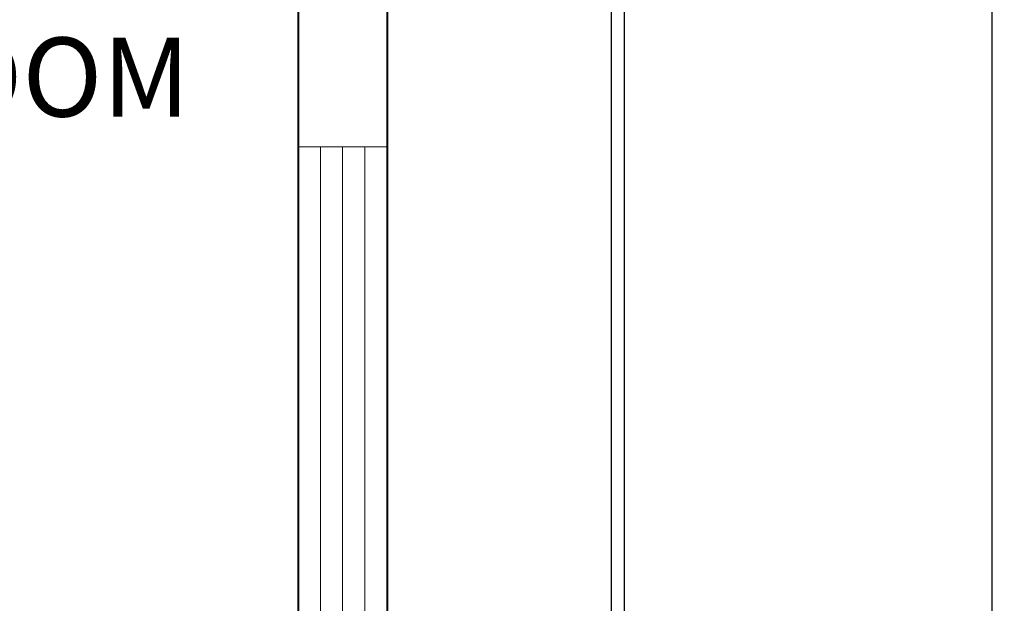
# Model space of a CAD drawing. Units: inches. Extents: x 459864 to 460310, y 324185 to 324787.
# Tile 109 of 112: x 460210 to 460310, y 324341 to 324400. Entities that reach past the tile are written whole.
import ezdxf

# ---------------------------------------------------------------- set-up
doc = ezdxf.new("R2010")
doc.units = ezdxf.units.IN
for name, color, linetype, lineweight in [('A-ANNO-DIMS', 2, 'Continuous', 18), ('A-AREA-IDEN', 7, 'Continuous', 25), ('A-GLAZ', 4, 'Continuous', 18), ('A-WALL', 7, 'Continuous', 40), ('C-PROP', 7, 'Continuous', 30)]:
    doc.layers.add(name, color=color, linetype=linetype, lineweight=lineweight)
doc.styles.get("Standard").update_dxf_attribs({"font": 'arial.ttf'})
doc.dimstyles.new('ISO-25', dxfattribs={"dimtxt": 6, "dimasz": 2.5, "dimexe": 1.25, "dimexo": 0.625, "dimtad": 1, "dimdec": 1, "dimlunit": 3, "dimtxsty": 'Standard', "dimcen": 2.5, "dimadec": 0, "dimazin": 0, "dimtfac": 1, "dimtdec": 1, "dimtmove": 0, "dimatfit": 3, "dimfxl": 1, "dimarcsym": 0})

# ---------------------------------------------------------------- blocks, each defined once
blk = doc.blocks.new('Window - Wood Frame 36 in. Wide plan')
for p, q in [((0, 6), (0, 0)), ((36, 6), (36, 0)), ((0, 4.5), (36, 4.5)), ((0, 3), (36, 3)), ((0, 1.5), (36, 1.5))]:
    blk.add_line(p, q)
blk = doc.blocks.new('*D21')
at = {"layer": 'A-ANNO-DIMS', "color": 0, "lineweight": -2, "transparency": 16777216}
for p, q in [((460247.74, 324715.483), (460309.58, 324715.483)), ((460308.33, 324712.983), (460308.33, 324285.983)), ((460247.74, 324283.483), (460309.58, 324283.483))]:
    blk.add_line(p, q, dxfattribs=at)
at = {"layer": 'A-ANNO-DIMS', "color": 0, "transparency": 16777216}
for points in [[(460307.914, 324712.983), (460308.747, 324712.983), (460308.33, 324715.483)], [(460307.914, 324285.983), (460308.747, 324285.983), (460308.33, 324283.483)]]:
    blk.add_solid(points, dxfattribs=at)
at = {"layer": 'Defpoints', "color": 0, "transparency": 16777216}
for p in [(460247.115, 324715.483), (460247.115, 324283.483), (460308.33, 324283.483)]:
    blk.add_point(p, dxfattribs=at)
at = {"layer": 'A-ANNO-DIMS', "color": 0, "transparency": 16777216, "insert": (460304.64, 324499.483), "char_height": 6, "attachment_point": 5, "rotation": 90}
blk.add_mtext("36'", dxfattribs=at)

msp = doc.modelspace()

# ---------------------------------------------------------------- linework, layer by layer
at = {"layer": 'A-WALL'}
for p, q in [((460247.115, 324470.983), (460247.115, 324283.483)), ((460238.115, 324466.483), (460238.115, 324292.483))]:
    msp.add_line(p, q, dxfattribs=at)
at = {"layer": 'C-PROP'}
for p, q in [((460269.804, 324466.483), (460269.804, 324199.483)), ((460271.115, 324466.483), (460271.115, 324194.947))]:
    msp.add_line(p, q, dxfattribs=at)

# ---------------------------------------------------------------- block references
at = {"layer": 'A-GLAZ', "xscale": 1.5, "yscale": 1.5, "zscale": 1.5, "rotation": 90}
msp.add_blockref('Window - Wood Frame 36 in. Wide plan', (460247.115, 324332.739), dxfattribs=at)

# ---------------------------------------------------------------- texts
at = {"layer": 'A-AREA-IDEN', "insert": (460127.286, 324397.798), "char_height": 8, "attachment_point": 1}
msp.add_mtext(' MASTER BEDROOM\\P12\'0"X12\'0"', dxfattribs=at)

# ---------------------------------------------------------------- dimensions: what is measured, and where the dimension line sits
at = {"layer": 'A-ANNO-DIMS'}
dim = msp.add_linear_dim(base=(460308.33, 324283.483), p1=(460247.115, 324715.483), p2=(460247.115, 324283.483), angle=90, dimstyle='ISO-25', override={"dimclrd": 0, "dimclre": 0, "dimclrt": 0}, dxfattribs=at)
dim.commit()
dim.dimension.update_dxf_attribs({"geometry": '*D21', "text_midpoint": (460304.64, 324499.483)})

doc.saveas('drawing.dxf')
